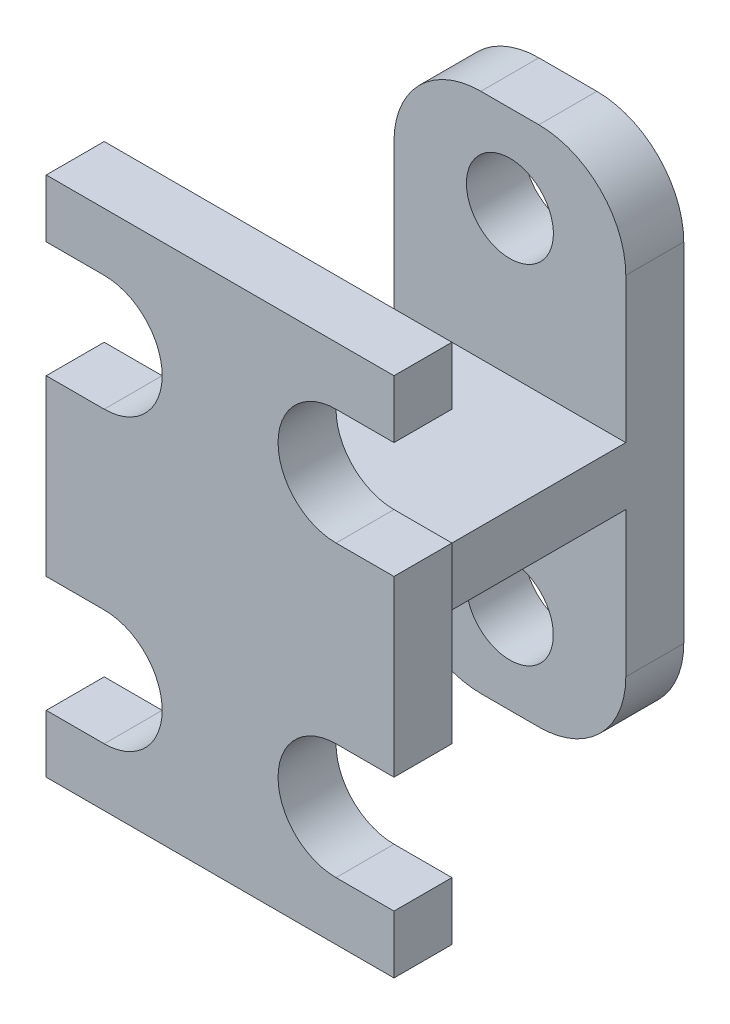
ISO-10303-21;
HEADER;
FILE_DESCRIPTION(('STEP AP214'),'2;1');
FILE_NAME('part.step','',(''),(''),'','','');
FILE_SCHEMA(('AUTOMOTIVE_DESIGN { 1 0 10303 214 1 1 1 1 }'));
ENDSEC;
DATA;
#1=APPLICATION_CONTEXT('core data for automotive mechanical design processes');
#2=APPLICATION_PROTOCOL_DEFINITION('international standard','automotive_design',2000,#1);
#3=PRODUCT_CONTEXT('',#1,'mechanical');
#4=PRODUCT('Part','Part','',(#3));
#5=PRODUCT_RELATED_PRODUCT_CATEGORY('part','',(#4));
#6=PRODUCT_DEFINITION_FORMATION('','',#4);
#7=PRODUCT_DEFINITION_CONTEXT('part definition',#1,'design');
#8=PRODUCT_DEFINITION('design','',#6,#7);
#9=PRODUCT_DEFINITION_SHAPE('','',#8);
#10=(LENGTH_UNIT() NAMED_UNIT(*) SI_UNIT(.MILLI.,.METRE.));
#11=(NAMED_UNIT(*) PLANE_ANGLE_UNIT() SI_UNIT($,.RADIAN.));
#12=(NAMED_UNIT(*) SI_UNIT($,.STERADIAN.) SOLID_ANGLE_UNIT());
#13=UNCERTAINTY_MEASURE_WITH_UNIT(LENGTH_MEASURE(1.E-05),#10,'distance_accuracy_value','');
#14=(GEOMETRIC_REPRESENTATION_CONTEXT(3) GLOBAL_UNCERTAINTY_ASSIGNED_CONTEXT((#13)) GLOBAL_UNIT_ASSIGNED_CONTEXT((#10,
#11,#12)) REPRESENTATION_CONTEXT('',''));
#15=CARTESIAN_POINT('',(0.,0.,0.));
#16=DIRECTION('',(0.,0.,1.));
#17=DIRECTION('',(1.,0.,0.));
#18=AXIS2_PLACEMENT_3D('',#15,#16,#17);
#19=CARTESIAN_POINT('',(5.00000000000001,2.,0.));
#20=DIRECTION('',(0.,0.,1.));
#21=DIRECTION('',(1.,0.,0.));
#22=AXIS2_PLACEMENT_3D('',#19,#20,#21);
#23=PLANE('',#22);
#24=DIRECTION('',(0.,-1.,0.));
#25=VECTOR('',#24,1.);
#26=CARTESIAN_POINT('',(0.,1.,0.));
#27=LINE('',#26,#25);
#28=CARTESIAN_POINT('',(0.,1.,0.));
#29=VERTEX_POINT('',#28);
#30=CARTESIAN_POINT('',(0.,0.,0.));
#31=VERTEX_POINT('',#30);
#32=EDGE_CURVE('E300',#29,#31,#27,.T.);
#33=ORIENTED_EDGE('',*,*,#32,.F.);
#34=DIRECTION('',(-1.,0.,0.));
#35=VECTOR('',#34,1.);
#36=CARTESIAN_POINT('',(1.,1.,0.));
#37=LINE('',#36,#35);
#38=CARTESIAN_POINT('',(1.,1.,0.));
#39=VERTEX_POINT('',#38);
#40=EDGE_CURVE('E305',#39,#29,#37,.T.);
#41=ORIENTED_EDGE('',*,*,#40,.F.);
#42=CARTESIAN_POINT('',(1.,2.,0.));
#43=DIRECTION('',(0.,0.,-1.));
#44=DIRECTION('',(-1.,0.,0.));
#45=AXIS2_PLACEMENT_3D('',#42,#43,#44);
#46=CIRCLE('',#45,1.);
#47=CARTESIAN_POINT('',(1.,3.,0.));
#48=VERTEX_POINT('',#47);
#49=EDGE_CURVE('E380',#48,#39,#46,.T.);
#50=ORIENTED_EDGE('',*,*,#49,.F.);
#51=DIRECTION('',(1.,0.,0.));
#52=VECTOR('',#51,1.);
#53=CARTESIAN_POINT('',(0.,3.,0.));
#54=LINE('',#53,#52);
#55=CARTESIAN_POINT('',(0.,3.,0.));
#56=VERTEX_POINT('',#55);
#57=EDGE_CURVE('E374',#56,#48,#54,.T.);
#58=ORIENTED_EDGE('',*,*,#57,.F.);
#59=DIRECTION('',(0.,-1.,0.));
#60=VECTOR('',#59,1.);
#61=CARTESIAN_POINT('',(0.,6.,0.));
#62=LINE('',#61,#60);
#63=CARTESIAN_POINT('',(0.,6.,0.));
#64=VERTEX_POINT('',#63);
#65=EDGE_CURVE('E373',#64,#56,#62,.T.);
#66=ORIENTED_EDGE('',*,*,#65,.F.);
#67=DIRECTION('',(-1.,0.,0.));
#68=VECTOR('',#67,1.);
#69=CARTESIAN_POINT('',(1.,6.,0.));
#70=LINE('',#69,#68);
#71=CARTESIAN_POINT('',(1.,6.,0.));
#72=VERTEX_POINT('',#71);
#73=EDGE_CURVE('E371',#72,#64,#70,.T.);
#74=ORIENTED_EDGE('',*,*,#73,.F.);
#75=CARTESIAN_POINT('',(1.,7.,0.));
#76=DIRECTION('',(0.,0.,-1.));
#77=DIRECTION('',(-1.,0.,0.));
#78=AXIS2_PLACEMENT_3D('',#75,#76,#77);
#79=CIRCLE('',#78,1.);
#80=CARTESIAN_POINT('',(1.,8.,0.));
#81=VERTEX_POINT('',#80);
#82=EDGE_CURVE('E367',#81,#72,#79,.T.);
#83=ORIENTED_EDGE('',*,*,#82,.F.);
#84=DIRECTION('',(1.,0.,0.));
#85=VECTOR('',#84,1.);
#86=CARTESIAN_POINT('',(0.,8.,0.));
#87=LINE('',#86,#85);
#88=CARTESIAN_POINT('',(0.,8.,0.));
#89=VERTEX_POINT('',#88);
#90=EDGE_CURVE('E370',#89,#81,#87,.T.);
#91=ORIENTED_EDGE('',*,*,#90,.F.);
#92=DIRECTION('',(0.,-1.,0.));
#93=VECTOR('',#92,1.);
#94=CARTESIAN_POINT('',(0.,9.,0.));
#95=LINE('',#94,#93);
#96=CARTESIAN_POINT('',(0.,9.,0.));
#97=VERTEX_POINT('',#96);
#98=EDGE_CURVE('E362',#97,#89,#95,.T.);
#99=ORIENTED_EDGE('',*,*,#98,.F.);
#100=DIRECTION('',(-1.,0.,0.));
#101=VECTOR('',#100,1.);
#102=CARTESIAN_POINT('',(6.,9.,0.));
#103=LINE('',#102,#101);
#104=CARTESIAN_POINT('',(6.,9.,0.));
#105=VERTEX_POINT('',#104);
#106=EDGE_CURVE('E361',#105,#97,#103,.T.);
#107=ORIENTED_EDGE('',*,*,#106,.F.);
#108=DIRECTION('',(0.,1.,0.));
#109=VECTOR('',#108,1.);
#110=CARTESIAN_POINT('',(6.,8.,0.));
#111=LINE('',#110,#109);
#112=CARTESIAN_POINT('',(6.,8.,0.));
#113=VERTEX_POINT('',#112);
#114=EDGE_CURVE('E363',#113,#105,#111,.T.);
#115=ORIENTED_EDGE('',*,*,#114,.F.);
#116=DIRECTION('',(1.,0.,0.));
#117=VECTOR('',#116,1.);
#118=CARTESIAN_POINT('',(6.,8.,0.));
#119=LINE('',#118,#117);
#120=CARTESIAN_POINT('',(5.,8.,0.));
#121=VERTEX_POINT('',#120);
#122=EDGE_CURVE('E360',#121,#113,#119,.T.);
#123=ORIENTED_EDGE('',*,*,#122,.F.);
#124=CARTESIAN_POINT('',(5.,7.,0.));
#125=DIRECTION('',(0.,0.,-1.));
#126=DIRECTION('',(1.,0.,0.));
#127=AXIS2_PLACEMENT_3D('',#124,#125,#126);
#128=CIRCLE('',#127,1.);
#129=CARTESIAN_POINT('',(5.,6.,0.));
#130=VERTEX_POINT('',#129);
#131=EDGE_CURVE('E357',#130,#121,#128,.T.);
#132=ORIENTED_EDGE('',*,*,#131,.F.);
#133=DIRECTION('',(-1.,0.,0.));
#134=VECTOR('',#133,1.);
#135=CARTESIAN_POINT('',(6.,6.,0.));
#136=LINE('',#135,#134);
#137=CARTESIAN_POINT('',(6.,6.,0.));
#138=VERTEX_POINT('',#137);
#139=EDGE_CURVE('E351',#138,#130,#136,.T.);
#140=ORIENTED_EDGE('',*,*,#139,.F.);
#141=DIRECTION('',(0.,1.,0.));
#142=VECTOR('',#141,1.);
#143=CARTESIAN_POINT('',(6.,3.,0.));
#144=LINE('',#143,#142);
#145=CARTESIAN_POINT('',(6.,3.,0.));
#146=VERTEX_POINT('',#145);
#147=EDGE_CURVE('E353',#146,#138,#144,.T.);
#148=ORIENTED_EDGE('',*,*,#147,.F.);
#149=DIRECTION('',(1.,0.,0.));
#150=VECTOR('',#149,1.);
#151=CARTESIAN_POINT('',(6.,3.,0.));
#152=LINE('',#151,#150);
#153=CARTESIAN_POINT('',(5.00000000000001,3.,0.));
#154=VERTEX_POINT('',#153);
#155=EDGE_CURVE('E352',#154,#146,#152,.T.);
#156=ORIENTED_EDGE('',*,*,#155,.F.);
#157=CARTESIAN_POINT('',(5.00000000000001,2.,0.));
#158=DIRECTION('',(0.,0.,-1.));
#159=DIRECTION('',(1.,0.,0.));
#160=AXIS2_PLACEMENT_3D('',#157,#158,#159);
#161=CIRCLE('',#160,1.);
#162=CARTESIAN_POINT('',(5.00000000000001,1.,0.));
#163=VERTEX_POINT('',#162);
#164=EDGE_CURVE('E347',#163,#154,#161,.T.);
#165=ORIENTED_EDGE('',*,*,#164,.F.);
#166=DIRECTION('',(-1.,0.,0.));
#167=VECTOR('',#166,1.);
#168=CARTESIAN_POINT('',(6.,1.,0.));
#169=LINE('',#168,#167);
#170=CARTESIAN_POINT('',(6.,1.,0.));
#171=VERTEX_POINT('',#170);
#172=EDGE_CURVE('E350',#171,#163,#169,.T.);
#173=ORIENTED_EDGE('',*,*,#172,.F.);
#174=DIRECTION('',(0.,1.,0.));
#175=VECTOR('',#174,1.);
#176=CARTESIAN_POINT('',(6.,0.,0.));
#177=LINE('',#176,#175);
#178=CARTESIAN_POINT('',(6.,0.,0.));
#179=VERTEX_POINT('',#178);
#180=EDGE_CURVE('E343',#179,#171,#177,.T.);
#181=ORIENTED_EDGE('',*,*,#180,.F.);
#182=DIRECTION('',(1.,0.,0.));
#183=VECTOR('',#182,1.);
#184=CARTESIAN_POINT('',(0.,0.,0.));
#185=LINE('',#184,#183);
#186=EDGE_CURVE('E344',#31,#179,#185,.T.);
#187=ORIENTED_EDGE('',*,*,#186,.F.);
#188=EDGE_LOOP('',(#33,#41,#50,#58,#66,#74,#83,#91,#99,#107,#115,#123,#132,#140,#148,#156,#165,
#173,#181,#187));
#189=FACE_BOUND('',#188,.T.);
#190=DIRECTION('',(0.,1.,0.));
#191=VECTOR('',#190,1.);
#192=CARTESIAN_POINT('',(1.,5.,0.));
#193=LINE('',#192,#191);
#194=CARTESIAN_POINT('',(1.,4.,0.));
#195=VERTEX_POINT('',#194);
#196=CARTESIAN_POINT('',(1.,5.,0.));
#197=VERTEX_POINT('',#196);
#198=EDGE_CURVE('E278',#195,#197,#193,.T.);
#199=ORIENTED_EDGE('',*,*,#198,.F.);
#200=DIRECTION('',(-1.,0.,0.));
#201=VECTOR('',#200,1.);
#202=CARTESIAN_POINT('',(5.,4.,0.));
#203=LINE('',#202,#201);
#204=CARTESIAN_POINT('',(5.,4.,0.));
#205=VERTEX_POINT('',#204);
#206=EDGE_CURVE('E268',#205,#195,#203,.T.);
#207=ORIENTED_EDGE('',*,*,#206,.F.);
#208=DIRECTION('',(0.,-1.,0.));
#209=VECTOR('',#208,1.);
#210=CARTESIAN_POINT('',(5.,5.,0.));
#211=LINE('',#210,#209);
#212=CARTESIAN_POINT('',(5.00000000000001,5.,0.));
#213=VERTEX_POINT('',#212);
#214=EDGE_CURVE('E287',#213,#205,#211,.T.);
#215=ORIENTED_EDGE('',*,*,#214,.F.);
#216=DIRECTION('',(1.,0.,0.));
#217=VECTOR('',#216,1.);
#218=CARTESIAN_POINT('',(5.,5.,0.));
#219=LINE('',#218,#217);
#220=EDGE_CURVE('E285',#197,#213,#219,.T.);
#221=ORIENTED_EDGE('',*,*,#220,.F.);
#222=EDGE_LOOP('',(#199,#207,#215,#221));
#223=FACE_BOUND('',#222,.T.);
#224=ADVANCED_FACE('F39',(#189,#223),#23,.F.);
#225=CARTESIAN_POINT('',(0.,1.,1.));
#226=DIRECTION('',(1.,0.,0.));
#227=DIRECTION('',(0.,0.,-1.));
#228=AXIS2_PLACEMENT_3D('',#225,#226,#227);
#229=PLANE('',#228);
#230=ORIENTED_EDGE('',*,*,#32,.T.);
#231=DIRECTION('',(0.,0.,-1.));
#232=VECTOR('',#231,1.);
#233=CARTESIAN_POINT('',(0.,0.,1.));
#234=LINE('',#233,#232);
#235=CARTESIAN_POINT('',(0.,0.,1.));
#236=VERTEX_POINT('',#235);
#237=EDGE_CURVE('E436',#236,#31,#234,.T.);
#238=ORIENTED_EDGE('',*,*,#237,.F.);
#239=DIRECTION('',(0.,-1.,0.));
#240=VECTOR('',#239,1.);
#241=CARTESIAN_POINT('',(0.,1.,1.));
#242=LINE('',#241,#240);
#243=CARTESIAN_POINT('',(0.,1.,1.));
#244=VERTEX_POINT('',#243);
#245=EDGE_CURVE('E296',#244,#236,#242,.T.);
#246=ORIENTED_EDGE('',*,*,#245,.F.);
#247=DIRECTION('',(0.,0.,-1.));
#248=VECTOR('',#247,1.);
#249=CARTESIAN_POINT('',(0.,1.,1.));
#250=LINE('',#249,#248);
#251=EDGE_CURVE('E338',#244,#29,#250,.T.);
#252=ORIENTED_EDGE('',*,*,#251,.T.);
#253=EDGE_LOOP('',(#230,#238,#246,#252));
#254=FACE_BOUND('',#253,.T.);
#255=ADVANCED_FACE('F522',(#254),#229,.F.);
#256=CARTESIAN_POINT('',(0.,0.,1.));
#257=DIRECTION('',(0.,1.,0.));
#258=DIRECTION('',(0.,0.,1.));
#259=AXIS2_PLACEMENT_3D('',#256,#257,#258);
#260=PLANE('',#259);
#261=ORIENTED_EDGE('',*,*,#186,.T.);
#262=DIRECTION('',(0.,0.,-1.));
#263=VECTOR('',#262,1.);
#264=CARTESIAN_POINT('',(6.,0.,1.));
#265=LINE('',#264,#263);
#266=CARTESIAN_POINT('',(6.,0.,1.));
#267=VERTEX_POINT('',#266);
#268=EDGE_CURVE('E433',#267,#179,#265,.T.);
#269=ORIENTED_EDGE('',*,*,#268,.F.);
#270=DIRECTION('',(1.,0.,0.));
#271=VECTOR('',#270,1.);
#272=CARTESIAN_POINT('',(0.,0.,1.));
#273=LINE('',#272,#271);
#274=EDGE_CURVE('E301',#236,#267,#273,.T.);
#275=ORIENTED_EDGE('',*,*,#274,.F.);
#276=ORIENTED_EDGE('',*,*,#237,.T.);
#277=EDGE_LOOP('',(#261,#269,#275,#276));
#278=FACE_BOUND('',#277,.T.);
#279=ADVANCED_FACE('F535',(#278),#260,.F.);
#280=CARTESIAN_POINT('',(6.,0.,1.));
#281=DIRECTION('',(-1.,0.,0.));
#282=DIRECTION('',(0.,0.,1.));
#283=AXIS2_PLACEMENT_3D('',#280,#281,#282);
#284=PLANE('',#283);
#285=ORIENTED_EDGE('',*,*,#180,.T.);
#286=DIRECTION('',(0.,0.,-1.));
#287=VECTOR('',#286,1.);
#288=CARTESIAN_POINT('',(6.,1.,1.));
#289=LINE('',#288,#287);
#290=CARTESIAN_POINT('',(6.,1.,1.));
#291=VERTEX_POINT('',#290);
#292=EDGE_CURVE('E427',#291,#171,#289,.T.);
#293=ORIENTED_EDGE('',*,*,#292,.F.);
#294=DIRECTION('',(0.,1.,0.));
#295=VECTOR('',#294,1.);
#296=CARTESIAN_POINT('',(6.,0.,1.));
#297=LINE('',#296,#295);
#298=EDGE_CURVE('E302',#267,#291,#297,.T.);
#299=ORIENTED_EDGE('',*,*,#298,.F.);
#300=ORIENTED_EDGE('',*,*,#268,.T.);
#301=EDGE_LOOP('',(#285,#293,#299,#300));
#302=FACE_BOUND('',#301,.T.);
#303=ADVANCED_FACE('F608',(#302),#284,.F.);
#304=CARTESIAN_POINT('',(6.,1.,1.));
#305=DIRECTION('',(0.,-1.,0.));
#306=DIRECTION('',(0.,0.,-1.));
#307=AXIS2_PLACEMENT_3D('',#304,#305,#306);
#308=PLANE('',#307);
#309=ORIENTED_EDGE('',*,*,#172,.T.);
#310=DIRECTION('',(0.,0.,-1.));
#311=VECTOR('',#310,1.);
#312=CARTESIAN_POINT('',(5.00000000000001,1.,1.));
#313=LINE('',#312,#311);
#314=CARTESIAN_POINT('',(5.00000000000001,1.,1.));
#315=VERTEX_POINT('',#314);
#316=EDGE_CURVE('E430',#315,#163,#313,.T.);
#317=ORIENTED_EDGE('',*,*,#316,.F.);
#318=DIRECTION('',(-1.,0.,0.));
#319=VECTOR('',#318,1.);
#320=CARTESIAN_POINT('',(6.,1.,1.));
#321=LINE('',#320,#319);
#322=EDGE_CURVE('E306',#291,#315,#321,.T.);
#323=ORIENTED_EDGE('',*,*,#322,.F.);
#324=ORIENTED_EDGE('',*,*,#292,.T.);
#325=EDGE_LOOP('',(#309,#317,#323,#324));
#326=FACE_BOUND('',#325,.T.);
#327=ADVANCED_FACE('F601',(#326),#308,.F.);
#328=CARTESIAN_POINT('',(5.00000000000001,2.,1.));
#329=DIRECTION('',(0.,0.,-1.));
#330=DIRECTION('',(-1.,0.,0.));
#331=AXIS2_PLACEMENT_3D('',#328,#329,#330);
#332=CYLINDRICAL_SURFACE('',#331,1.);
#333=ORIENTED_EDGE('',*,*,#164,.T.);
#334=DIRECTION('',(0.,0.,-1.));
#335=VECTOR('',#334,1.);
#336=CARTESIAN_POINT('',(5.00000000000001,3.,1.));
#337=LINE('',#336,#335);
#338=CARTESIAN_POINT('',(5.00000000000001,3.,1.));
#339=VERTEX_POINT('',#338);
#340=EDGE_CURVE('E425',#339,#154,#337,.T.);
#341=ORIENTED_EDGE('',*,*,#340,.F.);
#342=CARTESIAN_POINT('',(5.00000000000001,2.,1.));
#343=DIRECTION('',(0.,0.,-1.));
#344=DIRECTION('',(1.,0.,0.));
#345=AXIS2_PLACEMENT_3D('',#342,#343,#344);
#346=CIRCLE('',#345,1.);
#347=EDGE_CURVE('E308',#315,#339,#346,.T.);
#348=ORIENTED_EDGE('',*,*,#347,.F.);
#349=ORIENTED_EDGE('',*,*,#316,.T.);
#350=EDGE_LOOP('',(#333,#341,#348,#349));
#351=FACE_BOUND('',#350,.T.);
#352=ADVANCED_FACE('F598',(#351),#332,.F.);
#353=CARTESIAN_POINT('',(6.,3.,1.));
#354=DIRECTION('',(0.,1.,0.));
#355=DIRECTION('',(0.,0.,1.));
#356=AXIS2_PLACEMENT_3D('',#353,#354,#355);
#357=PLANE('',#356);
#358=ORIENTED_EDGE('',*,*,#155,.T.);
#359=DIRECTION('',(0.,0.,-1.));
#360=VECTOR('',#359,1.);
#361=CARTESIAN_POINT('',(6.,3.,1.));
#362=LINE('',#361,#360);
#363=CARTESIAN_POINT('',(6.,3.,1.));
#364=VERTEX_POINT('',#363);
#365=EDGE_CURVE('E423',#364,#146,#362,.T.);
#366=ORIENTED_EDGE('',*,*,#365,.F.);
#367=DIRECTION('',(1.,0.,0.));
#368=VECTOR('',#367,1.);
#369=CARTESIAN_POINT('',(6.,3.,1.));
#370=LINE('',#369,#368);
#371=EDGE_CURVE('E309',#339,#364,#370,.T.);
#372=ORIENTED_EDGE('',*,*,#371,.F.);
#373=ORIENTED_EDGE('',*,*,#340,.T.);
#374=EDGE_LOOP('',(#358,#366,#372,#373));
#375=FACE_BOUND('',#374,.T.);
#376=ADVANCED_FACE('F597',(#375),#357,.F.);
#377=CARTESIAN_POINT('',(6.,3.,1.));
#378=DIRECTION('',(-1.,0.,0.));
#379=DIRECTION('',(0.,0.,1.));
#380=AXIS2_PLACEMENT_3D('',#377,#378,#379);
#381=PLANE('',#380);
#382=ORIENTED_EDGE('',*,*,#147,.T.);
#383=DIRECTION('',(0.,0.,-1.));
#384=VECTOR('',#383,1.);
#385=CARTESIAN_POINT('',(6.,6.,1.));
#386=LINE('',#385,#384);
#387=CARTESIAN_POINT('',(6.,6.,1.));
#388=VERTEX_POINT('',#387);
#389=EDGE_CURVE('E418',#388,#138,#386,.T.);
#390=ORIENTED_EDGE('',*,*,#389,.F.);
#391=DIRECTION('',(0.,1.,0.));
#392=VECTOR('',#391,1.);
#393=CARTESIAN_POINT('',(6.,3.,1.));
#394=LINE('',#393,#392);
#395=EDGE_CURVE('E315',#364,#388,#394,.T.);
#396=ORIENTED_EDGE('',*,*,#395,.F.);
#397=ORIENTED_EDGE('',*,*,#365,.T.);
#398=EDGE_LOOP('',(#382,#390,#396,#397));
#399=FACE_BOUND('',#398,.T.);
#400=ADVANCED_FACE('F595',(#399),#381,.F.);
#401=CARTESIAN_POINT('',(6.,6.,1.));
#402=DIRECTION('',(0.,-1.,0.));
#403=DIRECTION('',(0.,0.,-1.));
#404=AXIS2_PLACEMENT_3D('',#401,#402,#403);
#405=PLANE('',#404);
#406=ORIENTED_EDGE('',*,*,#139,.T.);
#407=DIRECTION('',(0.,0.,-1.));
#408=VECTOR('',#407,1.);
#409=CARTESIAN_POINT('',(5.,6.,1.));
#410=LINE('',#409,#408);
#411=CARTESIAN_POINT('',(5.,6.,1.));
#412=VERTEX_POINT('',#411);
#413=EDGE_CURVE('E414',#412,#130,#410,.T.);
#414=ORIENTED_EDGE('',*,*,#413,.F.);
#415=DIRECTION('',(-1.,0.,0.));
#416=VECTOR('',#415,1.);
#417=CARTESIAN_POINT('',(6.,6.,1.));
#418=LINE('',#417,#416);
#419=EDGE_CURVE('E313',#388,#412,#418,.T.);
#420=ORIENTED_EDGE('',*,*,#419,.F.);
#421=ORIENTED_EDGE('',*,*,#389,.T.);
#422=EDGE_LOOP('',(#406,#414,#420,#421));
#423=FACE_BOUND('',#422,.T.);
#424=ADVANCED_FACE('F588',(#423),#405,.F.);
#425=CARTESIAN_POINT('',(5.,7.,1.));
#426=DIRECTION('',(0.,0.,-1.));
#427=DIRECTION('',(-1.,0.,0.));
#428=AXIS2_PLACEMENT_3D('',#425,#426,#427);
#429=CYLINDRICAL_SURFACE('',#428,1.);
#430=ORIENTED_EDGE('',*,*,#131,.T.);
#431=DIRECTION('',(0.,0.,-1.));
#432=VECTOR('',#431,1.);
#433=CARTESIAN_POINT('',(5.,8.,1.));
#434=LINE('',#433,#432);
#435=CARTESIAN_POINT('',(5.,8.,1.));
#436=VERTEX_POINT('',#435);
#437=EDGE_CURVE('E415',#436,#121,#434,.T.);
#438=ORIENTED_EDGE('',*,*,#437,.F.);
#439=CARTESIAN_POINT('',(5.,7.,1.));
#440=DIRECTION('',(0.,0.,-1.));
#441=DIRECTION('',(1.,0.,0.));
#442=AXIS2_PLACEMENT_3D('',#439,#440,#441);
#443=CIRCLE('',#442,1.);
#444=EDGE_CURVE('E317',#412,#436,#443,.T.);
#445=ORIENTED_EDGE('',*,*,#444,.F.);
#446=ORIENTED_EDGE('',*,*,#413,.T.);
#447=EDGE_LOOP('',(#430,#438,#445,#446));
#448=FACE_BOUND('',#447,.T.);
#449=ADVANCED_FACE('F581',(#448),#429,.F.);
#450=CARTESIAN_POINT('',(6.,8.,1.));
#451=DIRECTION('',(0.,1.,0.));
#452=DIRECTION('',(0.,0.,1.));
#453=AXIS2_PLACEMENT_3D('',#450,#451,#452);
#454=PLANE('',#453);
#455=ORIENTED_EDGE('',*,*,#122,.T.);
#456=DIRECTION('',(0.,0.,-1.));
#457=VECTOR('',#456,1.);
#458=CARTESIAN_POINT('',(6.,8.,1.));
#459=LINE('',#458,#457);
#460=CARTESIAN_POINT('',(6.,8.,1.));
#461=VERTEX_POINT('',#460);
#462=EDGE_CURVE('E406',#461,#113,#459,.T.);
#463=ORIENTED_EDGE('',*,*,#462,.F.);
#464=DIRECTION('',(1.,0.,0.));
#465=VECTOR('',#464,1.);
#466=CARTESIAN_POINT('',(6.,8.,1.));
#467=LINE('',#466,#465);
#468=EDGE_CURVE('E319',#436,#461,#467,.T.);
#469=ORIENTED_EDGE('',*,*,#468,.F.);
#470=ORIENTED_EDGE('',*,*,#437,.T.);
#471=EDGE_LOOP('',(#455,#463,#469,#470));
#472=FACE_BOUND('',#471,.T.);
#473=ADVANCED_FACE('F578',(#472),#454,.F.);
#474=CARTESIAN_POINT('',(6.,8.,1.));
#475=DIRECTION('',(-1.,0.,0.));
#476=DIRECTION('',(0.,0.,1.));
#477=AXIS2_PLACEMENT_3D('',#474,#475,#476);
#478=PLANE('',#477);
#479=ORIENTED_EDGE('',*,*,#114,.T.);
#480=DIRECTION('',(0.,0.,-1.));
#481=VECTOR('',#480,1.);
#482=CARTESIAN_POINT('',(6.,9.,1.));
#483=LINE('',#482,#481);
#484=CARTESIAN_POINT('',(6.,9.,1.));
#485=VERTEX_POINT('',#484);
#486=EDGE_CURVE('E407',#485,#105,#483,.T.);
#487=ORIENTED_EDGE('',*,*,#486,.F.);
#488=DIRECTION('',(0.,1.,0.));
#489=VECTOR('',#488,1.);
#490=CARTESIAN_POINT('',(6.,8.,1.));
#491=LINE('',#490,#489);
#492=EDGE_CURVE('E318',#461,#485,#491,.T.);
#493=ORIENTED_EDGE('',*,*,#492,.F.);
#494=ORIENTED_EDGE('',*,*,#462,.T.);
#495=EDGE_LOOP('',(#479,#487,#493,#494));
#496=FACE_BOUND('',#495,.T.);
#497=ADVANCED_FACE('F577',(#496),#478,.F.);
#498=CARTESIAN_POINT('',(6.,9.,1.));
#499=DIRECTION('',(0.,-1.,0.));
#500=DIRECTION('',(0.,0.,-1.));
#501=AXIS2_PLACEMENT_3D('',#498,#499,#500);
#502=PLANE('',#501);
#503=ORIENTED_EDGE('',*,*,#106,.T.);
#504=DIRECTION('',(0.,0.,-1.));
#505=VECTOR('',#504,1.);
#506=CARTESIAN_POINT('',(0.,9.,1.));
#507=LINE('',#506,#505);
#508=CARTESIAN_POINT('',(0.,9.,1.));
#509=VERTEX_POINT('',#508);
#510=EDGE_CURVE('E401',#509,#97,#507,.T.);
#511=ORIENTED_EDGE('',*,*,#510,.F.);
#512=DIRECTION('',(-1.,0.,0.));
#513=VECTOR('',#512,1.);
#514=CARTESIAN_POINT('',(6.,9.,1.));
#515=LINE('',#514,#513);
#516=EDGE_CURVE('E325',#485,#509,#515,.T.);
#517=ORIENTED_EDGE('',*,*,#516,.F.);
#518=ORIENTED_EDGE('',*,*,#486,.T.);
#519=EDGE_LOOP('',(#503,#511,#517,#518));
#520=FACE_BOUND('',#519,.T.);
#521=ADVANCED_FACE('F575',(#520),#502,.F.);
#522=CARTESIAN_POINT('',(0.,9.,1.));
#523=DIRECTION('',(1.,0.,0.));
#524=DIRECTION('',(0.,0.,-1.));
#525=AXIS2_PLACEMENT_3D('',#522,#523,#524);
#526=PLANE('',#525);
#527=ORIENTED_EDGE('',*,*,#98,.T.);
#528=DIRECTION('',(0.,0.,-1.));
#529=VECTOR('',#528,1.);
#530=CARTESIAN_POINT('',(0.,8.,1.));
#531=LINE('',#530,#529);
#532=CARTESIAN_POINT('',(0.,8.,1.));
#533=VERTEX_POINT('',#532);
#534=EDGE_CURVE('E396',#533,#89,#531,.T.);
#535=ORIENTED_EDGE('',*,*,#534,.F.);
#536=DIRECTION('',(0.,-1.,0.));
#537=VECTOR('',#536,1.);
#538=CARTESIAN_POINT('',(0.,9.,1.));
#539=LINE('',#538,#537);
#540=EDGE_CURVE('E321',#509,#533,#539,.T.);
#541=ORIENTED_EDGE('',*,*,#540,.F.);
#542=ORIENTED_EDGE('',*,*,#510,.T.);
#543=EDGE_LOOP('',(#527,#535,#541,#542));
#544=FACE_BOUND('',#543,.T.);
#545=ADVANCED_FACE('F568',(#544),#526,.F.);
#546=CARTESIAN_POINT('',(0.,8.,1.));
#547=DIRECTION('',(0.,1.,0.));
#548=DIRECTION('',(0.,0.,1.));
#549=AXIS2_PLACEMENT_3D('',#546,#547,#548);
#550=PLANE('',#549);
#551=ORIENTED_EDGE('',*,*,#90,.T.);
#552=DIRECTION('',(0.,0.,-1.));
#553=VECTOR('',#552,1.);
#554=CARTESIAN_POINT('',(1.,8.,1.));
#555=LINE('',#554,#553);
#556=CARTESIAN_POINT('',(1.,8.,1.));
#557=VERTEX_POINT('',#556);
#558=EDGE_CURVE('E400',#557,#81,#555,.T.);
#559=ORIENTED_EDGE('',*,*,#558,.F.);
#560=DIRECTION('',(1.,0.,0.));
#561=VECTOR('',#560,1.);
#562=CARTESIAN_POINT('',(0.,8.,1.));
#563=LINE('',#562,#561);
#564=EDGE_CURVE('E326',#533,#557,#563,.T.);
#565=ORIENTED_EDGE('',*,*,#564,.F.);
#566=ORIENTED_EDGE('',*,*,#534,.T.);
#567=EDGE_LOOP('',(#551,#559,#565,#566));
#568=FACE_BOUND('',#567,.T.);
#569=ADVANCED_FACE('F562',(#568),#550,.F.);
#570=CARTESIAN_POINT('',(1.,7.,1.));
#571=DIRECTION('',(0.,0.,-1.));
#572=DIRECTION('',(-1.,0.,0.));
#573=AXIS2_PLACEMENT_3D('',#570,#571,#572);
#574=CYLINDRICAL_SURFACE('',#573,1.);
#575=ORIENTED_EDGE('',*,*,#82,.T.);
#576=DIRECTION('',(0.,0.,-1.));
#577=VECTOR('',#576,1.);
#578=CARTESIAN_POINT('',(1.,6.,1.));
#579=LINE('',#578,#577);
#580=CARTESIAN_POINT('',(1.,6.,1.));
#581=VERTEX_POINT('',#580);
#582=EDGE_CURVE('E392',#581,#72,#579,.T.);
#583=ORIENTED_EDGE('',*,*,#582,.F.);
#584=CARTESIAN_POINT('',(1.,7.,1.));
#585=DIRECTION('',(0.,0.,-1.));
#586=DIRECTION('',(-1.,0.,0.));
#587=AXIS2_PLACEMENT_3D('',#584,#585,#586);
#588=CIRCLE('',#587,1.);
#589=EDGE_CURVE('E328',#557,#581,#588,.T.);
#590=ORIENTED_EDGE('',*,*,#589,.F.);
#591=ORIENTED_EDGE('',*,*,#558,.T.);
#592=EDGE_LOOP('',(#575,#583,#590,#591));
#593=FACE_BOUND('',#592,.T.);
#594=ADVANCED_FACE('F557',(#593),#574,.F.);
#595=CARTESIAN_POINT('',(1.,6.,1.));
#596=DIRECTION('',(0.,-1.,0.));
#597=DIRECTION('',(0.,0.,-1.));
#598=AXIS2_PLACEMENT_3D('',#595,#596,#597);
#599=PLANE('',#598);
#600=ORIENTED_EDGE('',*,*,#73,.T.);
#601=DIRECTION('',(0.,0.,-1.));
#602=VECTOR('',#601,1.);
#603=CARTESIAN_POINT('',(0.,6.,1.));
#604=LINE('',#603,#602);
#605=CARTESIAN_POINT('',(0.,6.,1.));
#606=VERTEX_POINT('',#605);
#607=EDGE_CURVE('E391',#606,#64,#604,.T.);
#608=ORIENTED_EDGE('',*,*,#607,.F.);
#609=DIRECTION('',(-1.,0.,0.));
#610=VECTOR('',#609,1.);
#611=CARTESIAN_POINT('',(1.,6.,1.));
#612=LINE('',#611,#610);
#613=EDGE_CURVE('E329',#581,#606,#612,.T.);
#614=ORIENTED_EDGE('',*,*,#613,.F.);
#615=ORIENTED_EDGE('',*,*,#582,.T.);
#616=EDGE_LOOP('',(#600,#608,#614,#615));
#617=FACE_BOUND('',#616,.T.);
#618=ADVANCED_FACE('F558',(#617),#599,.F.);
#619=CARTESIAN_POINT('',(0.,6.,1.));
#620=DIRECTION('',(1.,0.,0.));
#621=DIRECTION('',(0.,0.,-1.));
#622=AXIS2_PLACEMENT_3D('',#619,#620,#621);
#623=PLANE('',#622);
#624=ORIENTED_EDGE('',*,*,#65,.T.);
#625=DIRECTION('',(0.,0.,-1.));
#626=VECTOR('',#625,1.);
#627=CARTESIAN_POINT('',(0.,3.,1.));
#628=LINE('',#627,#626);
#629=CARTESIAN_POINT('',(0.,3.,1.));
#630=VERTEX_POINT('',#629);
#631=EDGE_CURVE('E389',#630,#56,#628,.T.);
#632=ORIENTED_EDGE('',*,*,#631,.F.);
#633=DIRECTION('',(0.,-1.,0.));
#634=VECTOR('',#633,1.);
#635=CARTESIAN_POINT('',(0.,6.,1.));
#636=LINE('',#635,#634);
#637=EDGE_CURVE('E335',#606,#630,#636,.T.);
#638=ORIENTED_EDGE('',*,*,#637,.F.);
#639=ORIENTED_EDGE('',*,*,#607,.T.);
#640=EDGE_LOOP('',(#624,#632,#638,#639));
#641=FACE_BOUND('',#640,.T.);
#642=ADVANCED_FACE('F552',(#641),#623,.F.);
#643=CARTESIAN_POINT('',(0.,3.,1.));
#644=DIRECTION('',(0.,1.,0.));
#645=DIRECTION('',(0.,0.,1.));
#646=AXIS2_PLACEMENT_3D('',#643,#644,#645);
#647=PLANE('',#646);
#648=ORIENTED_EDGE('',*,*,#57,.T.);
#649=DIRECTION('',(0.,0.,-1.));
#650=VECTOR('',#649,1.);
#651=CARTESIAN_POINT('',(1.,3.,1.));
#652=LINE('',#651,#650);
#653=CARTESIAN_POINT('',(1.,3.,1.));
#654=VERTEX_POINT('',#653);
#655=EDGE_CURVE('E383',#654,#48,#652,.T.);
#656=ORIENTED_EDGE('',*,*,#655,.F.);
#657=DIRECTION('',(1.,0.,0.));
#658=VECTOR('',#657,1.);
#659=CARTESIAN_POINT('',(0.,3.,1.));
#660=LINE('',#659,#658);
#661=EDGE_CURVE('E334',#630,#654,#660,.T.);
#662=ORIENTED_EDGE('',*,*,#661,.F.);
#663=ORIENTED_EDGE('',*,*,#631,.T.);
#664=EDGE_LOOP('',(#648,#656,#662,#663));
#665=FACE_BOUND('',#664,.T.);
#666=ADVANCED_FACE('F548',(#665),#647,.F.);
#667=CARTESIAN_POINT('',(1.,2.,1.));
#668=DIRECTION('',(0.,0.,-1.));
#669=DIRECTION('',(-1.,0.,0.));
#670=AXIS2_PLACEMENT_3D('',#667,#668,#669);
#671=CYLINDRICAL_SURFACE('',#670,1.);
#672=ORIENTED_EDGE('',*,*,#49,.T.);
#673=DIRECTION('',(0.,0.,-1.));
#674=VECTOR('',#673,1.);
#675=CARTESIAN_POINT('',(1.,1.,1.));
#676=LINE('',#675,#674);
#677=CARTESIAN_POINT('',(1.,1.,1.));
#678=VERTEX_POINT('',#677);
#679=EDGE_CURVE('E385',#678,#39,#676,.T.);
#680=ORIENTED_EDGE('',*,*,#679,.F.);
#681=CARTESIAN_POINT('',(1.,2.,1.));
#682=DIRECTION('',(0.,0.,-1.));
#683=DIRECTION('',(-1.,0.,0.));
#684=AXIS2_PLACEMENT_3D('',#681,#682,#683);
#685=CIRCLE('',#684,1.);
#686=EDGE_CURVE('E337',#654,#678,#685,.T.);
#687=ORIENTED_EDGE('',*,*,#686,.F.);
#688=ORIENTED_EDGE('',*,*,#655,.T.);
#689=EDGE_LOOP('',(#672,#680,#687,#688));
#690=FACE_BOUND('',#689,.T.);
#691=ADVANCED_FACE('F542',(#690),#671,.F.);
#692=CARTESIAN_POINT('',(1.,1.,1.));
#693=DIRECTION('',(0.,-1.,0.));
#694=DIRECTION('',(0.,0.,-1.));
#695=AXIS2_PLACEMENT_3D('',#692,#693,#694);
#696=PLANE('',#695);
#697=ORIENTED_EDGE('',*,*,#40,.T.);
#698=ORIENTED_EDGE('',*,*,#251,.F.);
#699=DIRECTION('',(-1.,0.,0.));
#700=VECTOR('',#699,1.);
#701=CARTESIAN_POINT('',(1.,1.,1.));
#702=LINE('',#701,#700);
#703=EDGE_CURVE('E336',#678,#244,#702,.T.);
#704=ORIENTED_EDGE('',*,*,#703,.F.);
#705=ORIENTED_EDGE('',*,*,#679,.T.);
#706=EDGE_LOOP('',(#697,#698,#704,#705));
#707=FACE_BOUND('',#706,.T.);
#708=ADVANCED_FACE('F541',(#707),#696,.F.);
#709=CARTESIAN_POINT('',(5.00000000000001,2.,1.));
#710=DIRECTION('',(0.,0.,1.));
#711=DIRECTION('',(1.,0.,0.));
#712=AXIS2_PLACEMENT_3D('',#709,#710,#711);
#713=PLANE('',#712);
#714=ORIENTED_EDGE('',*,*,#245,.T.);
#715=ORIENTED_EDGE('',*,*,#274,.T.);
#716=ORIENTED_EDGE('',*,*,#298,.T.);
#717=ORIENTED_EDGE('',*,*,#322,.T.);
#718=ORIENTED_EDGE('',*,*,#347,.T.);
#719=ORIENTED_EDGE('',*,*,#371,.T.);
#720=ORIENTED_EDGE('',*,*,#395,.T.);
#721=ORIENTED_EDGE('',*,*,#419,.T.);
#722=ORIENTED_EDGE('',*,*,#444,.T.);
#723=ORIENTED_EDGE('',*,*,#468,.T.);
#724=ORIENTED_EDGE('',*,*,#492,.T.);
#725=ORIENTED_EDGE('',*,*,#516,.T.);
#726=ORIENTED_EDGE('',*,*,#540,.T.);
#727=ORIENTED_EDGE('',*,*,#564,.T.);
#728=ORIENTED_EDGE('',*,*,#589,.T.);
#729=ORIENTED_EDGE('',*,*,#613,.T.);
#730=ORIENTED_EDGE('',*,*,#637,.T.);
#731=ORIENTED_EDGE('',*,*,#661,.T.);
#732=ORIENTED_EDGE('',*,*,#686,.T.);
#733=ORIENTED_EDGE('',*,*,#703,.T.);
#734=EDGE_LOOP('',(#714,#715,#716,#717,#718,#719,#720,#721,#722,#723,#724,#725,#726,#727,#728,
#729,#730,#731,#732,#733));
#735=FACE_BOUND('',#734,.T.);
#736=ADVANCED_FACE('F536',(#735),#713,.T.);
#737=CARTESIAN_POINT('',(1.,5.,-4.));
#738=DIRECTION('',(1.,0.,0.));
#739=DIRECTION('',(0.,0.,-1.));
#740=AXIS2_PLACEMENT_3D('',#737,#738,#739);
#741=PLANE('',#740);
#742=DIRECTION('',(0.,1.,0.));
#743=VECTOR('',#742,1.);
#744=CARTESIAN_POINT('',(1.,9.,-5.));
#745=LINE('',#744,#743);
#746=CARTESIAN_POINT('',(1.,1.5,-5.));
#747=VERTEX_POINT('',#746);
#748=CARTESIAN_POINT('',(1.,7.5,-5.));
#749=VERTEX_POINT('',#748);
#750=EDGE_CURVE('E483',#747,#749,#745,.T.);
#751=ORIENTED_EDGE('',*,*,#750,.F.);
#752=DIRECTION('',(0.,0.,1.));
#753=VECTOR('',#752,1.);
#754=CARTESIAN_POINT('',(1.,1.5,-4.));
#755=LINE('',#754,#753);
#756=CARTESIAN_POINT('',(1.,1.5,-4.));
#757=VERTEX_POINT('',#756);
#758=EDGE_CURVE('E253',#747,#757,#755,.T.);
#759=ORIENTED_EDGE('',*,*,#758,.T.);
#760=DIRECTION('',(0.,1.,0.));
#761=VECTOR('',#760,1.);
#762=CARTESIAN_POINT('',(1.,9.,-4.));
#763=LINE('',#762,#761);
#764=CARTESIAN_POINT('',(1.,4.,-4.));
#765=VERTEX_POINT('',#764);
#766=EDGE_CURVE('E247',#757,#765,#763,.T.);
#767=ORIENTED_EDGE('',*,*,#766,.T.);
#768=DIRECTION('',(0.,0.,1.));
#769=VECTOR('',#768,1.);
#770=CARTESIAN_POINT('',(1.,4.,-4.));
#771=LINE('',#770,#769);
#772=EDGE_CURVE('E254',#765,#195,#771,.T.);
#773=ORIENTED_EDGE('',*,*,#772,.T.);
#774=ORIENTED_EDGE('',*,*,#198,.T.);
#775=DIRECTION('',(0.,0.,1.));
#776=VECTOR('',#775,1.);
#777=CARTESIAN_POINT('',(1.,5.,-4.));
#778=LINE('',#777,#776);
#779=CARTESIAN_POINT('',(1.,5.,-4.));
#780=VERTEX_POINT('',#779);
#781=EDGE_CURVE('E295',#780,#197,#778,.T.);
#782=ORIENTED_EDGE('',*,*,#781,.F.);
#783=CARTESIAN_POINT('',(1.,7.5,-4.));
#784=VERTEX_POINT('',#783);
#785=EDGE_CURVE('E256',#780,#784,#763,.T.);
#786=ORIENTED_EDGE('',*,*,#785,.T.);
#787=DIRECTION('',(0.,0.,1.));
#788=VECTOR('',#787,1.);
#789=CARTESIAN_POINT('',(1.,7.5,-4.));
#790=LINE('',#789,#788);
#791=EDGE_CURVE('E437',#784,#749,#790,.F.);
#792=ORIENTED_EDGE('',*,*,#791,.T.);
#793=EDGE_LOOP('',(#751,#759,#767,#773,#774,#782,#786,#792));
#794=FACE_BOUND('',#793,.T.);
#795=ADVANCED_FACE('F252',(#794),#741,.F.);
#796=CARTESIAN_POINT('',(5.,5.,-4.));
#797=DIRECTION('',(0.,-1.,0.));
#798=DIRECTION('',(0.,0.,-1.));
#799=AXIS2_PLACEMENT_3D('',#796,#797,#798);
#800=PLANE('',#799);
#801=ORIENTED_EDGE('',*,*,#220,.T.);
#802=DIRECTION('',(0.,0.,1.));
#803=VECTOR('',#802,1.);
#804=CARTESIAN_POINT('',(5.,5.,-4.));
#805=LINE('',#804,#803);
#806=CARTESIAN_POINT('',(5.,5.,-4.));
#807=VERTEX_POINT('',#806);
#808=EDGE_CURVE('E293',#807,#213,#805,.T.);
#809=ORIENTED_EDGE('',*,*,#808,.F.);
#810=DIRECTION('',(1.,0.,0.));
#811=VECTOR('',#810,1.);
#812=CARTESIAN_POINT('',(5.,5.,-4.));
#813=LINE('',#812,#811);
#814=EDGE_CURVE('E274',#780,#807,#813,.T.);
#815=ORIENTED_EDGE('',*,*,#814,.F.);
#816=ORIENTED_EDGE('',*,*,#781,.T.);
#817=EDGE_LOOP('',(#801,#809,#815,#816));
#818=FACE_BOUND('',#817,.T.);
#819=ADVANCED_FACE('F629',(#818),#800,.F.);
#820=CARTESIAN_POINT('',(5.,5.,-4.));
#821=DIRECTION('',(-1.,0.,0.));
#822=DIRECTION('',(0.,-1.,0.));
#823=AXIS2_PLACEMENT_3D('',#820,#821,#822);
#824=PLANE('',#823);
#825=DIRECTION('',(0.,-1.,0.));
#826=VECTOR('',#825,1.);
#827=CARTESIAN_POINT('',(5.00000000000001,9.,-4.));
#828=LINE('',#827,#826);
#829=CARTESIAN_POINT('',(5.,4.,-4.));
#830=VERTEX_POINT('',#829);
#831=CARTESIAN_POINT('',(5.00000000000001,1.5,-4.));
#832=VERTEX_POINT('',#831);
#833=EDGE_CURVE('E271',#830,#832,#828,.T.);
#834=ORIENTED_EDGE('',*,*,#833,.T.);
#835=DIRECTION('',(0.,0.,1.));
#836=VECTOR('',#835,1.);
#837=CARTESIAN_POINT('',(5.,1.5,-4.));
#838=LINE('',#837,#836);
#839=CARTESIAN_POINT('',(5.00000000000001,1.5,-5.));
#840=VERTEX_POINT('',#839);
#841=EDGE_CURVE('E465',#832,#840,#838,.F.);
#842=ORIENTED_EDGE('',*,*,#841,.T.);
#843=DIRECTION('',(0.,-1.,0.));
#844=VECTOR('',#843,1.);
#845=CARTESIAN_POINT('',(5.00000000000001,9.,-5.));
#846=LINE('',#845,#844);
#847=CARTESIAN_POINT('',(5.00000000000001,7.5,-5.));
#848=VERTEX_POINT('',#847);
#849=EDGE_CURVE('E489',#848,#840,#846,.T.);
#850=ORIENTED_EDGE('',*,*,#849,.F.);
#851=DIRECTION('',(0.,0.,1.));
#852=VECTOR('',#851,1.);
#853=CARTESIAN_POINT('',(5.,7.5,-4.));
#854=LINE('',#853,#852);
#855=CARTESIAN_POINT('',(5.00000000000001,7.5,-4.));
#856=VERTEX_POINT('',#855);
#857=EDGE_CURVE('E457',#848,#856,#854,.T.);
#858=ORIENTED_EDGE('',*,*,#857,.T.);
#859=EDGE_CURVE('E478',#856,#807,#828,.T.);
#860=ORIENTED_EDGE('',*,*,#859,.T.);
#861=ORIENTED_EDGE('',*,*,#808,.T.);
#862=ORIENTED_EDGE('',*,*,#214,.T.);
#863=DIRECTION('',(0.,0.,1.));
#864=VECTOR('',#863,1.);
#865=CARTESIAN_POINT('',(5.,4.,-4.));
#866=LINE('',#865,#864);
#867=EDGE_CURVE('E269',#830,#205,#866,.T.);
#868=ORIENTED_EDGE('',*,*,#867,.F.);
#869=EDGE_LOOP('',(#834,#842,#850,#858,#860,#861,#862,#868));
#870=FACE_BOUND('',#869,.T.);
#871=ADVANCED_FACE('F507',(#870),#824,.F.);
#872=CARTESIAN_POINT('',(5.,4.,-4.));
#873=DIRECTION('',(0.,1.,0.));
#874=DIRECTION('',(0.,0.,1.));
#875=AXIS2_PLACEMENT_3D('',#872,#873,#874);
#876=PLANE('',#875);
#877=ORIENTED_EDGE('',*,*,#206,.T.);
#878=ORIENTED_EDGE('',*,*,#772,.F.);
#879=DIRECTION('',(-1.,0.,0.));
#880=VECTOR('',#879,1.);
#881=CARTESIAN_POINT('',(5.,4.,-4.));
#882=LINE('',#881,#880);
#883=EDGE_CURVE('E267',#830,#765,#882,.T.);
#884=ORIENTED_EDGE('',*,*,#883,.F.);
#885=ORIENTED_EDGE('',*,*,#867,.T.);
#886=EDGE_LOOP('',(#877,#878,#884,#885));
#887=FACE_BOUND('',#886,.T.);
#888=ADVANCED_FACE('F262',(#887),#876,.F.);
#889=CARTESIAN_POINT('',(0.,0.,-4.));
#890=DIRECTION('',(0.,0.,-1.));
#891=DIRECTION('',(-1.,0.,0.));
#892=AXIS2_PLACEMENT_3D('',#889,#890,#891);
#893=PLANE('',#892);
#894=CARTESIAN_POINT('',(3.,7.5,-4.));
#895=DIRECTION('',(0.,0.,-1.));
#896=DIRECTION('',(-1.,0.,0.));
#897=AXIS2_PLACEMENT_3D('',#894,#895,#896);
#898=CIRCLE('',#897,0.75);
#899=CARTESIAN_POINT('',(2.25,7.5,-4.));
#900=VERTEX_POINT('',#899);
#901=EDGE_CURVE('E631',#900,#900,#898,.T.);
#902=ORIENTED_EDGE('',*,*,#901,.T.);
#903=EDGE_LOOP('',(#902));
#904=FACE_BOUND('',#903,.T.);
#905=DIRECTION('',(1.,0.,0.));
#906=VECTOR('',#905,1.);
#907=CARTESIAN_POINT('',(5.00000000000001,9.,-4.));
#908=LINE('',#907,#906);
#909=CARTESIAN_POINT('',(2.5,9.,-4.));
#910=VERTEX_POINT('',#909);
#911=CARTESIAN_POINT('',(3.5,9.,-4.));
#912=VERTEX_POINT('',#911);
#913=EDGE_CURVE('E259',#910,#912,#908,.T.);
#914=ORIENTED_EDGE('',*,*,#913,.F.);
#915=CARTESIAN_POINT('',(2.5,7.5,-4.));
#916=DIRECTION('',(0.,0.,-1.));
#917=DIRECTION('',(-1.,0.,0.));
#918=AXIS2_PLACEMENT_3D('',#915,#916,#917);
#919=CIRCLE('',#918,1.5);
#920=EDGE_CURVE('E11',#910,#784,#919,.F.);
#921=ORIENTED_EDGE('',*,*,#920,.T.);
#922=ORIENTED_EDGE('',*,*,#785,.F.);
#923=ORIENTED_EDGE('',*,*,#814,.T.);
#924=ORIENTED_EDGE('',*,*,#859,.F.);
#925=CARTESIAN_POINT('',(3.5,7.5,-4.));
#926=DIRECTION('',(0.,0.,-1.));
#927=DIRECTION('',(-1.,0.,0.));
#928=AXIS2_PLACEMENT_3D('',#925,#926,#927);
#929=CIRCLE('',#928,1.5);
#930=EDGE_CURVE('E50',#856,#912,#929,.F.);
#931=ORIENTED_EDGE('',*,*,#930,.T.);
#932=EDGE_LOOP('',(#914,#921,#922,#923,#924,#931));
#933=FACE_BOUND('',#932,.T.);
#934=ADVANCED_FACE('F471',(#904,#933),#893,.F.);
#935=CARTESIAN_POINT('',(3.,1.5,-4.));
#936=DIRECTION('',(0.,0.,-1.));
#937=DIRECTION('',(-1.,0.,0.));
#938=AXIS2_PLACEMENT_3D('',#935,#936,#937);
#939=CIRCLE('',#938,0.749568333263736);
#940=CARTESIAN_POINT('',(2.25043166673626,1.5,-4.));
#941=VERTEX_POINT('',#940);
#942=EDGE_CURVE('E637',#941,#941,#939,.T.);
#943=ORIENTED_EDGE('',*,*,#942,.T.);
#944=EDGE_LOOP('',(#943));
#945=FACE_BOUND('',#944,.T.);
#946=ORIENTED_EDGE('',*,*,#766,.F.);
#947=CARTESIAN_POINT('',(2.5,1.5,-4.));
#948=DIRECTION('',(0.,0.,-1.));
#949=DIRECTION('',(-1.,0.,0.));
#950=AXIS2_PLACEMENT_3D('',#947,#948,#949);
#951=CIRCLE('',#950,1.5);
#952=CARTESIAN_POINT('',(2.5,0.,-4.));
#953=VERTEX_POINT('',#952);
#954=EDGE_CURVE('E443',#757,#953,#951,.F.);
#955=ORIENTED_EDGE('',*,*,#954,.T.);
#956=DIRECTION('',(-1.,0.,0.));
#957=VECTOR('',#956,1.);
#958=CARTESIAN_POINT('',(5.00000000000001,0.,-4.));
#959=LINE('',#958,#957);
#960=CARTESIAN_POINT('',(3.5,0.,-4.));
#961=VERTEX_POINT('',#960);
#962=EDGE_CURVE('E482',#961,#953,#959,.T.);
#963=ORIENTED_EDGE('',*,*,#962,.F.);
#964=CARTESIAN_POINT('',(3.5,1.5,-4.));
#965=DIRECTION('',(0.,0.,-1.));
#966=DIRECTION('',(-1.,0.,0.));
#967=AXIS2_PLACEMENT_3D('',#964,#965,#966);
#968=CIRCLE('',#967,1.5);
#969=EDGE_CURVE('E445',#961,#832,#968,.F.);
#970=ORIENTED_EDGE('',*,*,#969,.T.);
#971=ORIENTED_EDGE('',*,*,#833,.F.);
#972=ORIENTED_EDGE('',*,*,#883,.T.);
#973=EDGE_LOOP('',(#946,#955,#963,#970,#971,#972));
#974=FACE_BOUND('',#973,.T.);
#975=ADVANCED_FACE('F272',(#945,#974),#893,.F.);
#976=CARTESIAN_POINT('',(5.00000000000001,9.,-5.));
#977=DIRECTION('',(0.,-1.,0.));
#978=DIRECTION('',(0.,0.,-1.));
#979=AXIS2_PLACEMENT_3D('',#976,#977,#978);
#980=PLANE('',#979);
#981=DIRECTION('',(1.,0.,0.));
#982=VECTOR('',#981,1.);
#983=CARTESIAN_POINT('',(5.00000000000001,9.,-5.));
#984=LINE('',#983,#982);
#985=CARTESIAN_POINT('',(2.5,9.,-5.));
#986=VERTEX_POINT('',#985);
#987=CARTESIAN_POINT('',(3.5,9.,-5.));
#988=VERTEX_POINT('',#987);
#989=EDGE_CURVE('E475',#986,#988,#984,.T.);
#990=ORIENTED_EDGE('',*,*,#989,.F.);
#991=DIRECTION('',(0.,0.,1.));
#992=VECTOR('',#991,1.);
#993=CARTESIAN_POINT('',(2.5,9.,-5.));
#994=LINE('',#993,#992);
#995=EDGE_CURVE('E467',#986,#910,#994,.T.);
#996=ORIENTED_EDGE('',*,*,#995,.T.);
#997=ORIENTED_EDGE('',*,*,#913,.T.);
#998=DIRECTION('',(0.,0.,1.));
#999=VECTOR('',#998,1.);
#1000=CARTESIAN_POINT('',(3.5,9.,-5.));
#1001=LINE('',#1000,#999);
#1002=EDGE_CURVE('E464',#912,#988,#1001,.F.);
#1003=ORIENTED_EDGE('',*,*,#1002,.T.);
#1004=EDGE_LOOP('',(#990,#996,#997,#1003));
#1005=FACE_BOUND('',#1004,.T.);
#1006=ADVANCED_FACE('F469',(#1005),#980,.F.);
#1007=CARTESIAN_POINT('',(5.00000000000001,0.,-5.));
#1008=DIRECTION('',(0.,1.,0.));
#1009=DIRECTION('',(0.,0.,1.));
#1010=AXIS2_PLACEMENT_3D('',#1007,#1008,#1009);
#1011=PLANE('',#1010);
#1012=ORIENTED_EDGE('',*,*,#962,.T.);
#1013=DIRECTION('',(0.,0.,1.));
#1014=VECTOR('',#1013,1.);
#1015=CARTESIAN_POINT('',(2.5,0.,-5.));
#1016=LINE('',#1015,#1014);
#1017=CARTESIAN_POINT('',(2.5,0.,-5.));
#1018=VERTEX_POINT('',#1017);
#1019=EDGE_CURVE('E446',#953,#1018,#1016,.F.);
#1020=ORIENTED_EDGE('',*,*,#1019,.T.);
#1021=DIRECTION('',(-1.,0.,0.));
#1022=VECTOR('',#1021,1.);
#1023=CARTESIAN_POINT('',(5.00000000000001,0.,-5.));
#1024=LINE('',#1023,#1022);
#1025=CARTESIAN_POINT('',(3.5,0.,-5.));
#1026=VERTEX_POINT('',#1025);
#1027=EDGE_CURVE('E283',#1026,#1018,#1024,.T.);
#1028=ORIENTED_EDGE('',*,*,#1027,.F.);
#1029=DIRECTION('',(0.,0.,1.));
#1030=VECTOR('',#1029,1.);
#1031=CARTESIAN_POINT('',(3.5,0.,-5.));
#1032=LINE('',#1031,#1030);
#1033=EDGE_CURVE('E447',#1026,#961,#1032,.T.);
#1034=ORIENTED_EDGE('',*,*,#1033,.T.);
#1035=EDGE_LOOP('',(#1012,#1020,#1028,#1034));
#1036=FACE_BOUND('',#1035,.T.);
#1037=ADVANCED_FACE('F512',(#1036),#1011,.F.);
#1038=CARTESIAN_POINT('',(0.,0.,-5.));
#1039=DIRECTION('',(0.,0.,-1.));
#1040=DIRECTION('',(-1.,0.,0.));
#1041=AXIS2_PLACEMENT_3D('',#1038,#1039,#1040);
#1042=PLANE('',#1041);
#1043=CARTESIAN_POINT('',(3.,7.5,-5.));
#1044=DIRECTION('',(0.,0.,-1.));
#1045=DIRECTION('',(-1.,0.,0.));
#1046=AXIS2_PLACEMENT_3D('',#1043,#1044,#1045);
#1047=CIRCLE('',#1046,0.75);
#1048=CARTESIAN_POINT('',(2.25,7.5,-5.));
#1049=VERTEX_POINT('',#1048);
#1050=EDGE_CURVE('E633',#1049,#1049,#1047,.T.);
#1051=ORIENTED_EDGE('',*,*,#1050,.F.);
#1052=EDGE_LOOP('',(#1051));
#1053=FACE_BOUND('',#1052,.T.);
#1054=CARTESIAN_POINT('',(3.,1.5,-5.));
#1055=DIRECTION('',(0.,0.,-1.));
#1056=DIRECTION('',(-1.,0.,0.));
#1057=AXIS2_PLACEMENT_3D('',#1054,#1055,#1056);
#1058=CIRCLE('',#1057,0.749568333263736);
#1059=CARTESIAN_POINT('',(2.25043166673626,1.5,-5.));
#1060=VERTEX_POINT('',#1059);
#1061=EDGE_CURVE('E491',#1060,#1060,#1058,.T.);
#1062=ORIENTED_EDGE('',*,*,#1061,.F.);
#1063=EDGE_LOOP('',(#1062));
#1064=FACE_BOUND('',#1063,.T.);
#1065=ORIENTED_EDGE('',*,*,#1027,.T.);
#1066=CARTESIAN_POINT('',(2.5,1.5,-5.));
#1067=DIRECTION('',(0.,0.,-1.));
#1068=DIRECTION('',(-1.,0.,0.));
#1069=AXIS2_PLACEMENT_3D('',#1066,#1067,#1068);
#1070=CIRCLE('',#1069,1.5);
#1071=EDGE_CURVE('E460',#1018,#747,#1070,.T.);
#1072=ORIENTED_EDGE('',*,*,#1071,.T.);
#1073=ORIENTED_EDGE('',*,*,#750,.T.);
#1074=CARTESIAN_POINT('',(2.5,7.5,-5.));
#1075=DIRECTION('',(0.,0.,-1.));
#1076=DIRECTION('',(-1.,0.,0.));
#1077=AXIS2_PLACEMENT_3D('',#1074,#1075,#1076);
#1078=CIRCLE('',#1077,1.5);
#1079=EDGE_CURVE('E454',#749,#986,#1078,.T.);
#1080=ORIENTED_EDGE('',*,*,#1079,.T.);
#1081=ORIENTED_EDGE('',*,*,#989,.T.);
#1082=CARTESIAN_POINT('',(3.5,7.5,-5.));
#1083=DIRECTION('',(0.,0.,-1.));
#1084=DIRECTION('',(-1.,0.,0.));
#1085=AXIS2_PLACEMENT_3D('',#1082,#1083,#1084);
#1086=CIRCLE('',#1085,1.5);
#1087=EDGE_CURVE('E452',#988,#848,#1086,.T.);
#1088=ORIENTED_EDGE('',*,*,#1087,.T.);
#1089=ORIENTED_EDGE('',*,*,#849,.T.);
#1090=CARTESIAN_POINT('',(3.5,1.5,-5.));
#1091=DIRECTION('',(0.,0.,-1.));
#1092=DIRECTION('',(-1.,0.,0.));
#1093=AXIS2_PLACEMENT_3D('',#1090,#1091,#1092);
#1094=CIRCLE('',#1093,1.5);
#1095=EDGE_CURVE('E453',#840,#1026,#1094,.T.);
#1096=ORIENTED_EDGE('',*,*,#1095,.T.);
#1097=EDGE_LOOP('',(#1065,#1072,#1073,#1080,#1081,#1088,#1089,#1096));
#1098=FACE_BOUND('',#1097,.T.);
#1099=ADVANCED_FACE('F499',(#1053,#1064,#1098),#1042,.T.);
#1100=CARTESIAN_POINT('',(2.5,1.5,-4.));
#1101=DIRECTION('',(0.,0.,1.));
#1102=DIRECTION('',(1.,0.,0.));
#1103=AXIS2_PLACEMENT_3D('',#1100,#1101,#1102);
#1104=CYLINDRICAL_SURFACE('',#1103,1.5);
#1105=ORIENTED_EDGE('',*,*,#1071,.F.);
#1106=ORIENTED_EDGE('',*,*,#1019,.F.);
#1107=ORIENTED_EDGE('',*,*,#954,.F.);
#1108=ORIENTED_EDGE('',*,*,#758,.F.);
#1109=EDGE_LOOP('',(#1105,#1106,#1107,#1108));
#1110=FACE_BOUND('',#1109,.T.);
#1111=ADVANCED_FACE('F502',(#1110),#1104,.T.);
#1112=CARTESIAN_POINT('',(3.5,1.5,-5.));
#1113=DIRECTION('',(0.,0.,1.));
#1114=DIRECTION('',(1.,0.,0.));
#1115=AXIS2_PLACEMENT_3D('',#1112,#1113,#1114);
#1116=CYLINDRICAL_SURFACE('',#1115,1.5);
#1117=ORIENTED_EDGE('',*,*,#1095,.F.);
#1118=ORIENTED_EDGE('',*,*,#841,.F.);
#1119=ORIENTED_EDGE('',*,*,#969,.F.);
#1120=ORIENTED_EDGE('',*,*,#1033,.F.);
#1121=EDGE_LOOP('',(#1117,#1118,#1119,#1120));
#1122=FACE_BOUND('',#1121,.T.);
#1123=ADVANCED_FACE('F509',(#1122),#1116,.T.);
#1124=CARTESIAN_POINT('',(2.5,7.5,-5.));
#1125=DIRECTION('',(0.,0.,1.));
#1126=DIRECTION('',(1.,0.,0.));
#1127=AXIS2_PLACEMENT_3D('',#1124,#1125,#1126);
#1128=CYLINDRICAL_SURFACE('',#1127,1.5);
#1129=ORIENTED_EDGE('',*,*,#1079,.F.);
#1130=ORIENTED_EDGE('',*,*,#791,.F.);
#1131=ORIENTED_EDGE('',*,*,#920,.F.);
#1132=ORIENTED_EDGE('',*,*,#995,.F.);
#1133=EDGE_LOOP('',(#1129,#1130,#1131,#1132));
#1134=FACE_BOUND('',#1133,.T.);
#1135=ADVANCED_FACE('F616',(#1134),#1128,.T.);
#1136=CARTESIAN_POINT('',(3.5,7.5,-4.));
#1137=DIRECTION('',(0.,0.,1.));
#1138=DIRECTION('',(1.,0.,0.));
#1139=AXIS2_PLACEMENT_3D('',#1136,#1137,#1138);
#1140=CYLINDRICAL_SURFACE('',#1139,1.5);
#1141=ORIENTED_EDGE('',*,*,#1087,.F.);
#1142=ORIENTED_EDGE('',*,*,#1002,.F.);
#1143=ORIENTED_EDGE('',*,*,#930,.F.);
#1144=ORIENTED_EDGE('',*,*,#857,.F.);
#1145=EDGE_LOOP('',(#1141,#1142,#1143,#1144));
#1146=FACE_BOUND('',#1145,.T.);
#1147=ADVANCED_FACE('F41',(#1146),#1140,.T.);
#1148=CARTESIAN_POINT('',(3.,1.5,-4.));
#1149=DIRECTION('',(0.,0.,-1.));
#1150=DIRECTION('',(-1.,0.,0.));
#1151=AXIS2_PLACEMENT_3D('',#1148,#1149,#1150);
#1152=CYLINDRICAL_SURFACE('',#1151,0.749568333263736);
#1153=ORIENTED_EDGE('',*,*,#942,.F.);
#1154=EDGE_LOOP('',(#1153));
#1155=FACE_BOUND('',#1154,.T.);
#1156=ORIENTED_EDGE('',*,*,#1061,.T.);
#1157=EDGE_LOOP('',(#1156));
#1158=FACE_BOUND('',#1157,.T.);
#1159=ADVANCED_FACE('F621',(#1155,#1158),#1152,.F.);
#1160=CARTESIAN_POINT('',(3.,7.5,-4.));
#1161=DIRECTION('',(0.,0.,-1.));
#1162=DIRECTION('',(-1.,0.,0.));
#1163=AXIS2_PLACEMENT_3D('',#1160,#1161,#1162);
#1164=CYLINDRICAL_SURFACE('',#1163,0.75);
#1165=ORIENTED_EDGE('',*,*,#901,.F.);
#1166=EDGE_LOOP('',(#1165));
#1167=FACE_BOUND('',#1166,.T.);
#1168=ORIENTED_EDGE('',*,*,#1050,.T.);
#1169=EDGE_LOOP('',(#1168));
#1170=FACE_BOUND('',#1169,.T.);
#1171=ADVANCED_FACE('F649',(#1167,#1170),#1164,.F.);
#1172=CLOSED_SHELL('',(#224,#255,#279,#303,#327,#352,#376,#400,#424,#449,#473,#497,#521,#545,
#569,#594,#618,#642,#666,#691,#708,#736,#795,#819,#871,#888,#934,#975,#1006,#1037,#1099,#1111,
#1123,#1135,#1147,#1159,#1171));
#1173=MANIFOLD_SOLID_BREP('B2',#1172);
#1174=ADVANCED_BREP_SHAPE_REPRESENTATION('',(#18,#1173),#14);
#1175=SHAPE_DEFINITION_REPRESENTATION(#9,#1174);
ENDSEC;
END-ISO-10303-21;
